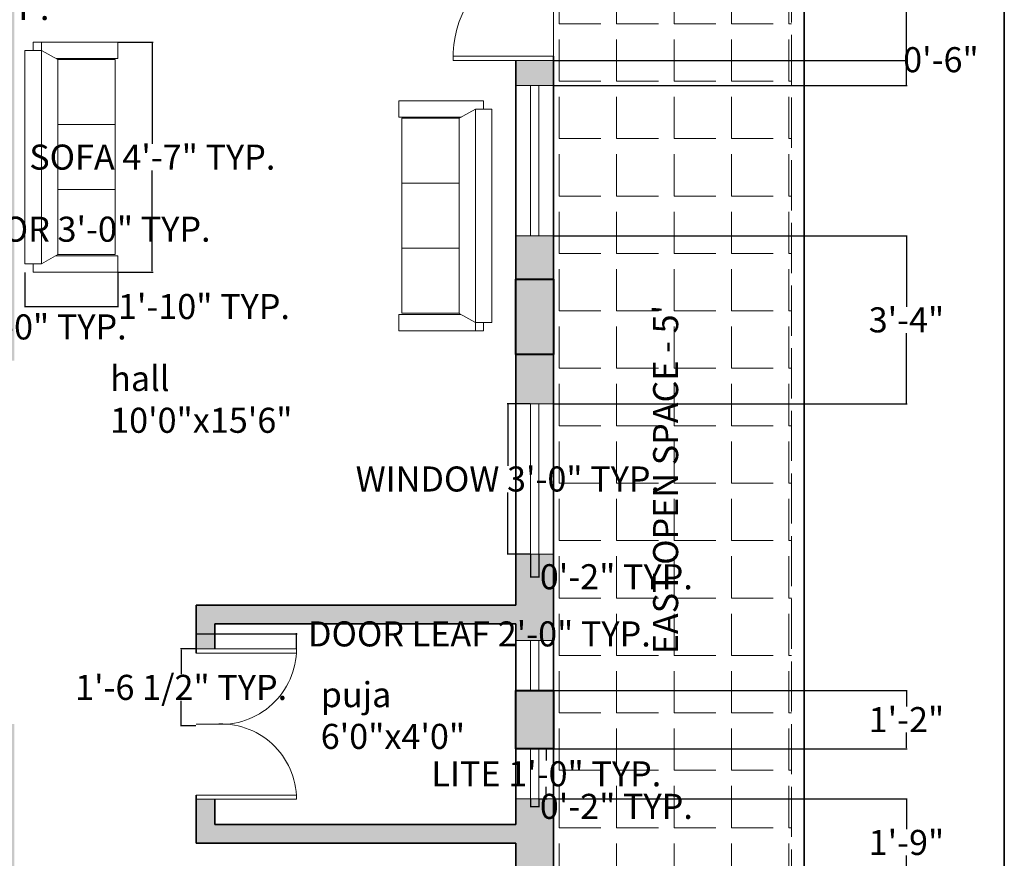
# Model space of a CAD drawing. Units: inches. Extents: x 56944 to 57417, y 173916 to 174454.
# Tile 6 of 8: x 57181 to 57417, y 174068 to 174268. Entities that reach past the tile are written whole.
import ezdxf

# ---------------------------------------------------------------- set-up
doc = ezdxf.new("R2010")
doc.units = ezdxf.units.IN
doc.header["$MEASUREMENT"] = 0
doc.linetypes.add('ACAD_ISO02W100', pattern=[15, 12, -3])
for name, color, linetype, lineweight in [('A-ANNO-DIMS', 2, 'Continuous', 18), ('A-ANNO-TEXT', 7, 'Continuous', 18), ('A-ANNO-TTLB', 7, 'Continuous', 35), ('A-AREA-IDEN', 7, 'Continuous', 20), ('A-COLS', 7, 'Continuous', 40), ('A-COLS-PATT', 250, 'Continuous', 9), ('A-DOOR', 3, 'Continuous', 20), ('A-FURN', 8, 'Continuous', 18), ('A-GLAZ', 4, 'Continuous', 18), ('A-SITE-PATT', 8, 'Continuous', 9), ('A-SITE-WALL-HIDN', 7, 'ACAD_ISO02W100', 18), ('A-WALL', 7, 'Continuous', 35), ('A-WALL-PATT', 241, 'Continuous', 9), ('C-PROP', 7, 'Continuous', 35)]:
    doc.layers.add(name, color=color, linetype=linetype, lineweight=lineweight)
doc.styles.get("Standard").update_dxf_attribs({"font": 'arial.ttf'})
doc.dimstyles.get("Standard").update_dxf_attribs({"dimtxt": 6, "dimasz": 0.18, "dimexe": 0.18, "dimexo": 0.0625, "dimgap": 0.09, "dimtad": 0, "dimtih": 1, "dimtoh": 1, "dimdec": 1, "dimzin": 0, "dimdsep": 46, "dimlunit": 3, "dimtxsty": 'Standard', "dimcen": 0.09, "dimadec": 0, "dimazin": 0, "dimtfac": 1, "dimtdec": 1, "dimtofl": 0, "dimtmove": 0, "dimatfit": 3, "dimfxl": 1, "dimtolj": 1, "dimtzin": 0, "dimarcsym": 0})

# ---------------------------------------------------------------- blocks, each defined once
blk = doc.blocks.new('SOFA-3-SEAT')
for p, q in [((1.96, 55.04), (22.23, 55.04)), ((1.96, 55.04), (1.96, 53.08)), ((3.92, 55.04), (3.92, 1.96)), ((22.23, 51.12), (22.23, 55.04)), ((0, 53.08), (0, 1.96)), ((3.92, 53.08), (0, 53.08)), ((3.92, 53.08), (7.85, 50.88)), ((7.54, 51.12), (22.23, 51.12)), ((21.57, 50.87), (7.85, 50.87)), ((21.57, 35.31), (7.85, 35.31)), ((21.57, 19.74), (7.85, 19.74)), ((7.85, 4.17), (3.92, 1.96)), ((7.28, 3.92), (22.23, 3.92)), ((22.23, 3.92), (22.23, 0)), ((3.92, 1.96), (0, 1.96)), ((1.96, 1.96), (1.96, 0)), ((1.96, 0), (22.23, 0))]:
    blk.add_line(p, q)
blk.add_lwpolyline([(7.85, 50.88), (7.85, 4.17), (21.57, 4.17), (21.57, 50.87)])
blk = doc.blocks.new('GLAZ-LITE-36IN')
for p, q in [((36, 2), (0, 2)), ((0, 0), (36, 0))]:
    blk.add_line(p, q)
blk = doc.blocks.new('GLAZ-LITE-12IN')
for p, q in [((0, 0), (0, 12)), ((2, 12), (2, 0))]:
    blk.add_line(p, q)
blk = doc.blocks.new('DOOR-PAIRED-LEAF-24IN')
for p, q in [((0, 18.06), (24, 18.06)), ((0, 18.06), (0, 17.06)), ((24, 17.06), (0, 17.06))]:
    blk.add_line(p, q)
blk.add_arc((5.94, 18.06), 18.06, 265.4188, 0)
blk = doc.blocks.new('*D14')
at = {"layer": 'A-ANNO-DIMS', "color": 0, "lineweight": -2, "transparency": 16777216}
for p, q in [((57303.07, 174176.51), (57297.55, 174176.51)), ((57297.73, 174176.33), (57297.73, 174161.7)), ((57297.73, 174140.69), (57297.73, 174155.31)), ((57303.07, 174140.51), (57297.55, 174140.51))]:
    blk.add_line(p, q, dxfattribs=at)
at = {"layer": 'A-ANNO-DIMS', "color": 0, "transparency": 16777216}
for points in [[(57297.7, 174176.33), (57297.76, 174176.33), (57297.73, 174176.51)], [(57297.7, 174140.69), (57297.76, 174140.69), (57297.73, 174140.51)]]:
    blk.add_solid(points, dxfattribs=at)
at = {"layer": 'Defpoints', "color": 0, "transparency": 16777216}
for p in [(57303.13, 174176.51), (57297.73, 174140.51), (57303.13, 174140.51)]:
    blk.add_point(p, dxfattribs=at)
at = {"layer": 'A-ANNO-DIMS', "color": 0, "transparency": 16777216, "insert": (57297.73, 174158.51), "char_height": 6, "attachment_point": 5}
blk.add_mtext('\\A1;WINDOW 3\'-0" TYP.', dxfattribs=at)
blk = doc.blocks.new('*D15')
at = {"layer": 'A-ANNO-DIMS', "color": 0, "lineweight": -2, "transparency": 16777216}
for p, q in [((57303.13, 174140.44), (57303.13, 174134.93)), ((57305.13, 174140.44), (57305.13, 174134.93)), ((57303.31, 174135.11), (57304.95, 174135.11)), ((57305.13, 174135.11), (57305.31, 174135.11))]:
    blk.add_line(p, q, dxfattribs=at)
at = {"layer": 'A-ANNO-DIMS', "color": 0, "transparency": 16777216}
for points in [[(57303.31, 174135.14), (57303.31, 174135.08), (57303.13, 174135.11)], [(57304.95, 174135.14), (57304.95, 174135.08), (57305.13, 174135.11)]]:
    blk.add_solid(points, dxfattribs=at)
at = {"layer": 'Defpoints', "color": 0, "transparency": 16777216}
for p in [(57303.13, 174140.51), (57305.13, 174140.51), (57305.13, 174135.11)]:
    blk.add_point(p, dxfattribs=at)
at = {"layer": 'A-ANNO-DIMS', "color": 0, "transparency": 16777216, "insert": (57323.69, 174135.11), "char_height": 6, "attachment_point": 5}
blk.add_mtext('\\A1;0\'-2" TYP.', dxfattribs=at)
blk = doc.blocks.new('*D16')
at = {"layer": 'A-ANNO-DIMS', "color": 0, "lineweight": -2, "transparency": 16777216}
for p, q in [((57135.34, 174305.75), (57145.76, 174305.75)), ((57145.58, 174305.57), (57145.58, 174274.59)), ((57145.58, 174237.22), (57145.58, 174268.2)), ((57135.34, 174237.04), (57145.76, 174237.04))]:
    blk.add_line(p, q, dxfattribs=at)
at = {"layer": 'A-ANNO-DIMS', "color": 0, "transparency": 16777216}
for points in [[(57145.55, 174305.57), (57145.61, 174305.57), (57145.58, 174305.75)], [(57145.55, 174237.22), (57145.61, 174237.22), (57145.58, 174237.04)]]:
    blk.add_solid(points, dxfattribs=at)
at = {"layer": 'Defpoints', "color": 0, "transparency": 16777216}
for p in [(57135.28, 174305.75), (57145.58, 174305.75), (57135.28, 174237.04)]:
    blk.add_point(p, dxfattribs=at)
at = {"layer": 'A-ANNO-DIMS', "color": 0, "transparency": 16777216, "insert": (57145.58, 174271.39), "char_height": 6, "attachment_point": 5}
blk.add_mtext('\\A1;BED SET 5\'-8 1/2" TYP.', dxfattribs=at)
blk = doc.blocks.new('*D18')
at = {"layer": 'A-ANNO-DIMS', "color": 0, "lineweight": -2, "transparency": 16777216}
for p, q in [((57204.45, 174263.1), (57212.82, 174263.1)), ((57212.64, 174262.92), (57212.64, 174238.77)), ((57212.64, 174208.24), (57212.64, 174232.38)), ((57204.45, 174208.06), (57212.82, 174208.06))]:
    blk.add_line(p, q, dxfattribs=at)
at = {"layer": 'A-ANNO-DIMS', "color": 0, "transparency": 16777216}
for points in [[(57212.61, 174262.92), (57212.67, 174262.92), (57212.64, 174263.1)], [(57212.61, 174208.24), (57212.67, 174208.24), (57212.64, 174208.06)]]:
    blk.add_solid(points, dxfattribs=at)
at = {"layer": 'Defpoints', "color": 0, "transparency": 16777216}
for p in [(57204.39, 174263.1), (57212.64, 174263.1), (57204.39, 174208.06)]:
    blk.add_point(p, dxfattribs=at)
at = {"layer": 'A-ANNO-DIMS', "color": 0, "transparency": 16777216, "insert": (57212.64, 174235.58), "char_height": 6, "attachment_point": 5}
blk.add_mtext('\\A1;SOFA 4\'-7" TYP.', dxfattribs=at)
blk = doc.blocks.new('*D19')
at = {"layer": 'A-ANNO-DIMS', "color": 0, "lineweight": -2, "transparency": 16777216}
for p, q in [((57182.16, 174207.99), (57182.16, 174199.62)), ((57204.39, 174207.99), (57204.39, 174199.62)), ((57182.34, 174199.8), (57204.21, 174199.8)), ((57204.39, 174199.8), (57204.57, 174199.8))]:
    blk.add_line(p, q, dxfattribs=at)
at = {"layer": 'A-ANNO-DIMS', "color": 0, "transparency": 16777216}
for points in [[(57182.34, 174199.83), (57182.34, 174199.77), (57182.16, 174199.8)], [(57204.21, 174199.83), (57204.21, 174199.77), (57204.39, 174199.8)]]:
    blk.add_solid(points, dxfattribs=at)
at = {"layer": 'Defpoints', "color": 0, "transparency": 16777216}
for p in [(57182.16, 174208.06), (57204.39, 174208.06), (57204.39, 174199.8)]:
    blk.add_point(p, dxfattribs=at)
at = {"layer": 'A-ANNO-DIMS', "color": 0, "transparency": 16777216, "insert": (57224.99, 174199.8), "char_height": 6, "attachment_point": 5}
blk.add_mtext('\\A1;1\'-10" TYP.', dxfattribs=at)
blk = doc.blocks.new('*D22')
at = {"layer": 'A-ANNO-DIMS', "color": 0, "lineweight": -2, "transparency": 16777216}
for p, q in [((57169.7, 174236.32), (57175.21, 174236.32)), ((57175.03, 174236.14), (57175.03, 174221.52)), ((57175.03, 174200.5), (57175.03, 174215.13)), ((57169.7, 174200.32), (57175.21, 174200.32))]:
    blk.add_line(p, q, dxfattribs=at)
at = {"layer": 'A-ANNO-DIMS', "color": 0, "transparency": 16777216}
for points in [[(57175, 174236.14), (57175.06, 174236.14), (57175.03, 174236.32)], [(57175, 174200.5), (57175.06, 174200.5), (57175.03, 174200.32)]]:
    blk.add_solid(points, dxfattribs=at)
at = {"layer": 'Defpoints', "color": 0, "transparency": 16777216}
for p in [(57169.63, 174236.32), (57175.03, 174236.32), (57169.63, 174200.32)]:
    blk.add_point(p, dxfattribs=at)
at = {"layer": 'A-ANNO-DIMS', "color": 0, "transparency": 16777216, "insert": (57175.03, 174218.32), "char_height": 6, "attachment_point": 5}
blk.add_mtext('\\A1;BEDROOM DOOR 3\'-0" TYP.', dxfattribs=at)
blk = doc.blocks.new('*D23')
at = {"layer": 'A-ANNO-DIMS', "color": 0, "lineweight": -2, "transparency": 16777216}
for p, q in [((57133.63, 174200.26), (57133.63, 174194.74)), ((57169.63, 174200.26), (57169.63, 174194.74)), ((57133.81, 174194.92), (57169.45, 174194.92)), ((57169.63, 174194.92), (57169.81, 174194.92))]:
    blk.add_line(p, q, dxfattribs=at)
at = {"layer": 'A-ANNO-DIMS', "color": 0, "transparency": 16777216}
for points in [[(57133.81, 174194.95), (57133.81, 174194.89), (57133.63, 174194.92)], [(57169.45, 174194.95), (57169.45, 174194.89), (57169.63, 174194.92)]]:
    blk.add_solid(points, dxfattribs=at)
at = {"layer": 'Defpoints', "color": 0, "transparency": 16777216}
for p in [(57133.63, 174200.32), (57169.63, 174200.32), (57169.63, 174194.92)]:
    blk.add_point(p, dxfattribs=at)
at = {"layer": 'A-ANNO-DIMS', "color": 0, "transparency": 16777216, "insert": (57188.19, 174194.92), "char_height": 6, "attachment_point": 5}
blk.add_mtext('\\A1;3\'-0" TYP.', dxfattribs=at)
blk = doc.blocks.new('*D28')
at = {"layer": 'A-ANNO-DIMS', "color": 0, "lineweight": -2, "transparency": 16777216}
for p, q in [((57305.2, 174093.93), (57307.11, 174093.93)), ((57306.93, 174093.75), (57306.93, 174091.08)), ((57306.93, 174082.11), (57306.93, 174084.78)), ((57305.2, 174081.93), (57307.11, 174081.93))]:
    blk.add_line(p, q, dxfattribs=at)
at = {"layer": 'A-ANNO-DIMS', "color": 0, "transparency": 16777216}
for points in [[(57306.9, 174093.75), (57306.96, 174093.75), (57306.93, 174093.93)], [(57306.9, 174082.11), (57306.96, 174082.11), (57306.93, 174081.93)]]:
    blk.add_solid(points, dxfattribs=at)
at = {"layer": 'Defpoints', "color": 0, "transparency": 16777216}
for p in [(57305.13, 174093.93), (57306.93, 174093.93), (57305.13, 174081.93)]:
    blk.add_point(p, dxfattribs=at)
at = {"layer": 'A-ANNO-DIMS', "color": 0, "transparency": 16777216, "insert": (57306.93, 174087.93), "char_height": 6, "attachment_point": 5}
blk.add_mtext('\\A1;LITE 1\'-0" TYP.', dxfattribs=at)
blk = doc.blocks.new('*D29')
at = {"layer": 'A-ANNO-DIMS', "color": 0, "lineweight": -2, "transparency": 16777216}
for p, q in [((57303.13, 174081.87), (57303.13, 174079.95)), ((57303.31, 174080.13), (57304.95, 174080.13)), ((57305.13, 174081.87), (57305.13, 174079.95)), ((57305.13, 174080.13), (57305.31, 174080.13))]:
    blk.add_line(p, q, dxfattribs=at)
at = {"layer": 'A-ANNO-DIMS', "color": 0, "transparency": 16777216}
for points in [[(57303.31, 174080.16), (57303.31, 174080.1), (57303.13, 174080.13)], [(57304.95, 174080.16), (57304.95, 174080.1), (57305.13, 174080.13)]]:
    blk.add_solid(points, dxfattribs=at)
at = {"layer": 'Defpoints', "color": 0, "transparency": 16777216}
for p in [(57303.13, 174081.93), (57305.13, 174081.93), (57305.13, 174080.13)]:
    blk.add_point(p, dxfattribs=at)
at = {"layer": 'A-ANNO-DIMS', "color": 0, "transparency": 16777216, "insert": (57323.69, 174080.13), "char_height": 6, "attachment_point": 5}
blk.add_mtext('\\A1;0\'-2" TYP.', dxfattribs=at)
blk = doc.blocks.new('*D30')
at = {"layer": 'A-ANNO-DIMS', "color": 0, "lineweight": -2, "transparency": 16777216}
for p, q in [((57223.13, 174117.89), (57223.13, 174121.6)), ((57223.31, 174121.42), (57246.95, 174121.42)), ((57247.13, 174117.89), (57247.13, 174121.6)), ((57247.13, 174121.42), (57247.31, 174121.42))]:
    blk.add_line(p, q, dxfattribs=at)
at = {"layer": 'A-ANNO-DIMS', "color": 0, "transparency": 16777216}
for points in [[(57223.31, 174121.45), (57223.31, 174121.39), (57223.13, 174121.42)], [(57246.95, 174121.45), (57246.95, 174121.39), (57247.13, 174121.42)]]:
    blk.add_solid(points, dxfattribs=at)
at = {"layer": 'Defpoints', "color": 0, "transparency": 16777216}
for p in [(57247.13, 174121.42), (57223.13, 174117.82), (57247.13, 174117.82)]:
    blk.add_point(p, dxfattribs=at)
at = {"layer": 'A-ANNO-DIMS', "color": 0, "transparency": 16777216, "insert": (57290.92, 174121.42), "char_height": 6, "attachment_point": 5}
blk.add_mtext('\\A1;DOOR LEAF 2\'-0" TYP.', dxfattribs=at)
blk = doc.blocks.new('*D31')
at = {"layer": 'A-ANNO-DIMS', "color": 0, "lineweight": -2, "transparency": 16777216}
for p, q in [((57223.07, 174117.82), (57219.35, 174117.82)), ((57219.53, 174117.64), (57219.53, 174111.81)), ((57219.53, 174099.6), (57219.53, 174105.43)), ((57223.07, 174099.42), (57219.35, 174099.42))]:
    blk.add_line(p, q, dxfattribs=at)
at = {"layer": 'A-ANNO-DIMS', "color": 0, "transparency": 16777216}
for points in [[(57219.5, 174117.64), (57219.56, 174117.64), (57219.53, 174117.82)], [(57219.5, 174099.6), (57219.56, 174099.6), (57219.53, 174099.42)]]:
    blk.add_solid(points, dxfattribs=at)
at = {"layer": 'Defpoints', "color": 0, "transparency": 16777216}
for p in [(57219.53, 174117.82), (57223.13, 174117.82), (57223.13, 174099.42)]:
    blk.add_point(p, dxfattribs=at)
at = {"layer": 'A-ANNO-DIMS', "color": 0, "transparency": 16777216, "insert": (57219.53, 174108.62), "char_height": 6, "attachment_point": 5}
blk.add_mtext('\\A1;1\'-6 1/2" TYP.', dxfattribs=at)
blk = doc.blocks.new('*D45')
at = {"layer": 'A-ANNO-DIMS', "color": 0, "lineweight": -2, "transparency": 16777216}
for p, q in [((57308.7, 174306.82), (57393.31, 174306.82)), ((57393.13, 174306.64), (57393.13, 174285.93)), ((57393.13, 174258.9), (57393.13, 174279.62)), ((57308.7, 174258.72), (57393.31, 174258.72))]:
    blk.add_line(p, q, dxfattribs=at)
at = {"layer": 'A-ANNO-DIMS', "color": 0, "transparency": 16777216}
for points in [[(57393.1, 174306.64), (57393.16, 174306.64), (57393.13, 174306.82)], [(57393.1, 174258.9), (57393.16, 174258.9), (57393.13, 174258.72)]]:
    blk.add_solid(points, dxfattribs=at)
at = {"layer": 'Defpoints', "color": 0, "transparency": 16777216}
for p in [(57308.63, 174306.82), (57393.13, 174306.82), (57308.63, 174258.72)]:
    blk.add_point(p, dxfattribs=at)
at = {"layer": 'A-ANNO-DIMS', "color": 0, "transparency": 16777216, "insert": (57393.13, 174282.77), "char_height": 6, "attachment_point": 5}
blk.add_mtext('\\A1;4\'-0"', dxfattribs=at)
blk = doc.blocks.new('*D50')
at = {"layer": 'A-ANNO-DIMS', "color": 0, "lineweight": -2, "transparency": 16777216}
for p, q in [((57308.7, 174081.93), (57393.31, 174081.93)), ((57393.13, 174081.75), (57393.13, 174074.65)), ((57393.13, 174061.23), (57393.13, 174068.34)), ((57308.7, 174061.05), (57393.31, 174061.05))]:
    blk.add_line(p, q, dxfattribs=at)
at = {"layer": 'A-ANNO-DIMS', "color": 0, "transparency": 16777216}
for points in [[(57393.1, 174081.75), (57393.16, 174081.75), (57393.13, 174081.93)], [(57393.1, 174061.23), (57393.16, 174061.23), (57393.13, 174061.05)]]:
    blk.add_solid(points, dxfattribs=at)
at = {"layer": 'Defpoints', "color": 0, "transparency": 16777216}
for p in [(57308.63, 174081.93), (57393.13, 174081.93), (57308.63, 174061.05)]:
    blk.add_point(p, dxfattribs=at)
at = {"layer": 'A-ANNO-DIMS', "color": 0, "transparency": 16777216, "insert": (57393.13, 174071.49), "char_height": 6, "attachment_point": 5}
blk.add_mtext('\\A1;1\'-9"', dxfattribs=at)
blk = doc.blocks.new('*D51')
at = {"layer": 'A-ANNO-DIMS', "color": 0, "lineweight": -2, "transparency": 16777216}
for p, q in [((57308.7, 174107.87), (57393.31, 174107.87)), ((57393.13, 174107.69), (57393.13, 174104)), ((57393.13, 174094.11), (57393.13, 174097.8)), ((57308.7, 174093.93), (57393.31, 174093.93))]:
    blk.add_line(p, q, dxfattribs=at)
at = {"layer": 'A-ANNO-DIMS', "color": 0, "transparency": 16777216}
for points in [[(57393.1, 174107.69), (57393.16, 174107.69), (57393.13, 174107.87)], [(57393.1, 174094.11), (57393.16, 174094.11), (57393.13, 174093.93)]]:
    blk.add_solid(points, dxfattribs=at)
at = {"layer": 'Defpoints', "color": 0, "transparency": 16777216}
for p in [(57308.63, 174107.87), (57393.13, 174107.87), (57308.63, 174093.93)]:
    blk.add_point(p, dxfattribs=at)
at = {"layer": 'A-ANNO-DIMS', "color": 0, "transparency": 16777216, "insert": (57393.13, 174100.9), "char_height": 6, "attachment_point": 5}
blk.add_mtext('\\A1;1\'-2"', dxfattribs=at)
blk = doc.blocks.new('*D52')
at = {"layer": 'A-ANNO-DIMS', "color": 0, "lineweight": -2, "transparency": 16777216}
for p, q in [((57308.7, 174258.72), (57393.31, 174258.72)), ((57393.13, 174258.72), (57393.13, 174258.9)), ((57393.13, 174258.9), (57393.31, 174258.9)), ((57393.13, 174252.9), (57393.13, 174258.54)), ((57308.7, 174252.72), (57393.31, 174252.72))]:
    blk.add_line(p, q, dxfattribs=at)
at = {"layer": 'A-ANNO-DIMS', "color": 0, "transparency": 16777216}
for points in [[(57393.1, 174258.54), (57393.16, 174258.54), (57393.13, 174258.72)], [(57393.1, 174252.9), (57393.16, 174252.9), (57393.13, 174252.72)]]:
    blk.add_solid(points, dxfattribs=at)
at = {"layer": 'Defpoints', "color": 0, "transparency": 16777216}
for p in [(57308.63, 174258.72), (57393.13, 174258.72), (57308.63, 174252.72)]:
    blk.add_point(p, dxfattribs=at)
at = {"layer": 'A-ANNO-DIMS', "color": 0, "transparency": 16777216, "insert": (57401.38, 174258.9), "char_height": 6, "attachment_point": 5}
blk.add_mtext('\\A1;0\'-6"', dxfattribs=at)
blk = doc.blocks.new('*D53')
at = {"layer": 'A-ANNO-DIMS', "color": 0, "lineweight": -2, "transparency": 16777216}
for p, q in [((57308.7, 174216.72), (57393.31, 174216.72)), ((57393.13, 174216.54), (57393.13, 174199.77)), ((57393.13, 174176.69), (57393.13, 174193.46)), ((57308.7, 174176.51), (57393.31, 174176.51))]:
    blk.add_line(p, q, dxfattribs=at)
at = {"layer": 'A-ANNO-DIMS', "color": 0, "transparency": 16777216}
for points in [[(57393.1, 174216.54), (57393.16, 174216.54), (57393.13, 174216.72)], [(57393.1, 174176.69), (57393.16, 174176.69), (57393.13, 174176.51)]]:
    blk.add_solid(points, dxfattribs=at)
at = {"layer": 'Defpoints', "color": 0, "transparency": 16777216}
for p in [(57308.63, 174216.72), (57393.13, 174216.72), (57308.63, 174176.51)]:
    blk.add_point(p, dxfattribs=at)
at = {"layer": 'A-ANNO-DIMS', "color": 0, "transparency": 16777216, "insert": (57393.13, 174196.61), "char_height": 6, "attachment_point": 5}
blk.add_mtext('\\A1;3\'-4"', dxfattribs=at)

msp = doc.modelspace()

# ---------------------------------------------------------------- hatches: boundary and pattern name
at = {"layer": 'A-COLS-PATT'}
h = msp.add_hatch(color=256, dxfattribs=at)
h.dxf.hatch_style = 1
h.paths.add_polyline_path([(57052.13, 174321.82), (57034.13, 174321.82), (57034.13, 174312.82), (57052.13, 174312.82)])
h.paths.add_polyline_path([(57186.38, 174321.82), (57168.38, 174321.82), (57168.38, 174312.82), (57175.13, 174312.82), (57186.38, 174312.82)])
h.paths.add_polyline_path([(57308.63, 174321.82), (57290.63, 174321.82), (57290.63, 174312.82), (57308.63, 174312.82)])
h.paths.add_polyline_path([(57179.63, 174204.82), (57170.63, 174204.82), (57170.63, 174186.82), (57179.63, 174186.82)])
h.paths.add_polyline_path([(57043.13, 174204.82), (57034.13, 174204.82), (57034.13, 174186.82), (57043.13, 174186.82)])
h.paths.add_polyline_path([(57308.63, 174206.32), (57299.63, 174206.32), (57299.63, 174188.32), (57308.63, 174188.32)])
h.paths.add_polyline_path([(57308.63, 174107.87), (57299.63, 174107.87), (57299.63, 174093.93), (57308.63, 174093.93)])
h.paths.add_polyline_path([(57308.63, 173978.32), (57299.63, 173978.32), (57299.63, 173960.32), (57308.63, 173960.32)])
h.paths.add_polyline_path([(57179.63, 173969.32), (57161.63, 173969.32), (57161.63, 173960.32), (57179.63, 173960.32)])
h.paths.add_polyline_path([(57043.13, 173978.32), (57034.13, 173978.32), (57034.13, 173960.32), (57043.13, 173960.32)])
h.paths.add_polyline_path([(57043.13, 174099.82), (57034.13, 174099.82), (57034.13, 174081.82), (57043.13, 174081.82)])
h.paths.add_polyline_path([(57179.63, 174099.82), (57170.63, 174099.82), (57170.63, 174081.82), (57179.63, 174081.82)])
at = {"layer": 'A-SITE-PATT'}
h = msp.add_hatch(dxfattribs=at)
h.set_pattern_fill('ANGLE', color=256, scale=50)
h.set_pattern_definition([(0, (0, 0), (0, 13.75), [10, -3.75]), (90, (0, 0), (-13.75, 8e-16), [10, -3.75])])
h.paths.add_polyline_path([(57365.63, 174396.82), (57200.13, 174396.82), (57200.13, 174379.18), (57215.46, 174379.18, -1.049383), (57218.84, 174379.34, -0.952941), (57215.46, 174379.18), (57200.13, 174379.18), (57200.13, 174360.82), (57140.13, 174360.82), (57140.13, 174321.82), (57149.42, 174321.82), (57243.2, 174321.82), (57282.32, 174321.82), (57283.32, 174321.82), (57308.63, 174321.82), (57308.63, 174305.82), (57308.63, 174259.72), (57308.63, 174258.72), (57308.63, 174252.72), (57308.63, 174216.72), (57308.63, 174099.82), (57308.63, 174093.93), (57308.63, 174081.93), (57308.63, 173969.32), (57365.63, 173969.32)])
h.paths.add_polyline_path([(57341.88, 174114.38), (57341.88, 174209.81), (57329.51, 174209.81), (57329.51, 174114.38)], flags=24)
h.paths.add_polyline_path([(57215.63, 174350.61), (57326.6, 174350.61), (57326.6, 174362.97), (57215.63, 174362.97)], flags=24)
at = {"layer": 'A-WALL-PATT'}
h = msp.add_hatch(color=256, dxfattribs=at)
h.dxf.hatch_style = 1
h.paths.add_polyline_path([(57089.42, 174321.82), (57052.13, 174321.82), (57052.13, 174312.82), (57089.42, 174312.82)])
h.paths.add_polyline_path([(57168.38, 174321.82), (57149.42, 174321.82), (57149.42, 174312.82), (57168.38, 174312.82)])
h.paths.add_polyline_path([(57199.66, 174321.82), (57186.38, 174321.82), (57186.38, 174312.82), (57199.66, 174312.82)])
h.paths.add_polyline_path([(57179.63, 174312.82), (57177.38, 174312.82), (57175.13, 174312.82), (57175.13, 174204.82), (57179.63, 174204.82)])
h.paths.add_polyline_path([(57043.13, 174312.82), (57034.13, 174312.82), (57034.13, 174204.82), (57043.13, 174204.82)])
h.paths.add_polyline_path([(57043.13, 174147.82), (57121.13, 174147.82), (57121.13, 174099.82), (57115.13, 174099.82), (57115.13, 174095.32), (57121.13, 174095.32), (57133.63, 174095.32), (57133.63, 174099.82), (57125.63, 174099.82), (57125.63, 174200.32), (57133.63, 174200.32), (57133.63, 174204.82), (57115.13, 174204.82), (57115.13, 174200.32), (57121.13, 174200.32), (57121.13, 174152.32), (57043.13, 174152.32), (57043.13, 174162.82), (57034.13, 174162.82), (57034.13, 174131.11), (57043.13, 174131.11)])
h.paths.add_polyline_path([(57043.13, 174081.82), (57034.13, 174081.82), (57034.13, 173978.32), (57043.13, 173978.32)])
h.paths.add_polyline_path([(57093.93, 173969.32), (57043.13, 173969.32), (57043.13, 173960.32), (57093.93, 173960.32)])
h.paths.add_polyline_path([(57161.63, 173969.32), (57153.93, 173969.32), (57153.93, 173960.32), (57161.63, 173960.32)])
h.paths.add_polyline_path([(57179.63, 174081.82), (57175.13, 174081.82), (57175.13, 173969.32), (57179.63, 173969.32)])
h.paths.add_polyline_path([(57299.63, 173969.32), (57179.63, 173969.32), (57179.63, 173960.32), (57299.63, 173960.32)])
h.paths.add_polyline_path([(57308.63, 174025.05), (57299.63, 174025.05), (57299.63, 173978.32), (57308.63, 173978.32)])
h.paths.add_polyline_path([(57308.63, 174081.93), (57299.63, 174081.93), (57299.63, 174075.82), (57227.63, 174075.82), (57227.63, 174081.82), (57223.13, 174081.82), (57223.13, 174075.82), (57223.13, 174071.32), (57299.63, 174071.32), (57299.63, 174061.05), (57308.63, 174061.05)])
h.paths.add_polyline_path([(57308.63, 174140.51), (57299.63, 174140.51), (57299.63, 174128.32), (57223.13, 174128.32), (57223.13, 174117.82), (57227.63, 174117.82), (57227.63, 174123.82), (57299.63, 174123.82), (57299.63, 174119.87), (57308.63, 174119.87)])
h.paths.add_polyline_path([(57308.63, 174216.72), (57299.63, 174216.72), (57299.63, 174206.32), (57308.63, 174206.32)])
h.paths.add_polyline_path([(57308.63, 174188.32), (57299.63, 174188.32), (57299.63, 174176.51), (57308.63, 174176.51)])
h.paths.add_polyline_path([(57308.63, 174258.72), (57299.63, 174258.72), (57299.63, 174252.72), (57308.63, 174252.72)])
h.paths.add_polyline_path([(57308.63, 174312.82), (57299.63, 174312.82), (57299.63, 174306.82), (57308.63, 174306.82)])
h.paths.add_polyline_path([(57290.63, 174321.82), (57283.32, 174321.82), (57283.32, 174312.82), (57290.63, 174312.82)])
h.paths.add_polyline_path([(57242.2, 174321.82), (57235.66, 174321.82), (57235.66, 174312.82), (57242.2, 174312.82)])
h.paths.add_polyline_path([(57083.13, 174204.82), (57043.13, 174204.82), (57043.13, 174200.32), (57083.13, 174200.32)], flags=17)
h.paths.add_polyline_path([(57083.13, 174099.82), (57043.13, 174099.82), (57043.13, 174095.32), (57083.13, 174095.32)], flags=0)

# ---------------------------------------------------------------- linework, layer by layer
at = {"layer": 'A-ANNO-TTLB'}
msp.add_lwpolyline([(56943.57, 174453.61), (57416.55, 174453.61), (57416.55, 173915.6), (56943.57, 173915.6)], close=True, dxfattribs=at)
at = {"layer": 'A-COLS'}
for p, q in [((57299.63, 174206.32), (57308.63, 174206.32)), ((57299.63, 174188.32), (57299.63, 174206.32)), ((57308.63, 174206.32), (57308.63, 174188.32)), ((57308.63, 174188.32), (57299.63, 174188.32)), ((57299.63, 174107.87), (57308.63, 174107.87)), ((57299.63, 174093.93), (57299.63, 174107.87)), ((57308.63, 174107.87), (57308.63, 174093.93)), ((57308.63, 174093.93), (57299.63, 174093.93)), ((57299.63, 174093.93), (57299.63, 174093.93))]:
    msp.add_line(p, q, dxfattribs=at)
at = {"layer": 'A-DOOR'}
for p, q in [((57308.63, 174305.82), (57308.63, 174259.72)), ((57284.63, 174259.72), (57308.63, 174259.72)), ((57308.63, 174258.72), (57308.63, 174259.72)), ((57308.63, 174258.72), (57284.63, 174258.72)), ((57284.63, 174258.72), (57308.63, 174258.72)), ((57247.13, 174117.82), (57223.13, 174117.82)), ((57223.13, 174116.82), (57223.13, 174117.82)), ((57223.13, 174099.82), (57227.63, 174099.82)), ((57247.13, 174081.82), (57223.13, 174081.82))]:
    msp.add_line(p, q, dxfattribs=at)
msp.add_arc((57310.15, 174259.51), 25.53, 114.3285, 181.7674, dxfattribs=at)
at = {"layer": 'A-GLAZ'}
for p, q in [((57308.63, 174252.72), (57299.63, 174252.72)), ((57299.63, 174252.72), (57299.63, 174216.72)), ((57308.63, 174216.72), (57308.63, 174252.72)), ((57299.63, 174216.72), (57308.63, 174216.72)), ((57299.63, 174140.51), (57299.63, 174176.51)), ((57299.63, 174176.51), (57308.63, 174176.51)), ((57308.63, 174176.51), (57308.63, 174140.51)), ((57308.63, 174140.51), (57299.63, 174140.51)), ((57299.63, 174107.87), (57299.63, 174119.87)), ((57299.63, 174119.87), (57308.63, 174119.87)), ((57308.63, 174119.87), (57308.63, 174107.87)), ((57308.63, 174107.87), (57299.63, 174107.87)), ((57299.63, 174093.93), (57308.63, 174093.93)), ((57299.63, 174081.93), (57299.63, 174093.93)), ((57308.63, 174093.93), (57308.63, 174081.93)), ((57308.63, 174081.93), (57299.63, 174081.93))]:
    msp.add_line(p, q, dxfattribs=at)
at = {"layer": 'A-SITE-WALL-HIDN'}
msp.add_line((57365.63, 174399.82), (57365.63, 173969.32), dxfattribs=at)
at = {"layer": 'A-WALL'}
for p, q in [((57308.63, 174259.72), (57308.63, 174099.82)), ((57299.63, 174258.72), (57299.63, 174128.32)), ((57308.63, 174252.72), (57308.63, 174258.72)), ((57223.13, 174128.32), (57223.13, 174116.82)), ((57223.13, 174128.32), (57299.63, 174128.32)), ((57223.13, 174123.82), (57223.13, 174117.82)), ((57227.63, 174123.82), (57227.63, 174117.82)), ((57227.63, 174123.82), (57299.63, 174123.82)), ((57299.63, 174123.82), (57299.63, 174099.82)), ((57299.63, 174099.82), (57299.63, 174075.82)), ((57308.63, 174099.82), (57308.63, 173960.32)), ((57223.13, 174082.82), (57223.13, 174071.32)), ((57223.13, 174075.82), (57223.13, 174081.82)), ((57227.63, 174081.82), (57227.63, 174075.82)), ((57227.63, 174075.82), (57299.63, 174075.82)), ((57223.13, 174071.32), (57299.63, 174071.32)), ((57299.63, 174071.32), (57299.63, 173960.32))]:
    msp.add_line(p, q, dxfattribs=at)
at = {"layer": 'C-PROP'}
msp.add_line((57368.63, 174399.82), (57368.63, 173960.32), dxfattribs=at)

# ---------------------------------------------------------------- block references
at = {"layer": 'A-DOOR'}
msp.add_blockref('DOOR-PAIRED-LEAF-24IN', (57223.13, 174099.77), dxfattribs=at)
at = {"layer": 'A-DOOR', "extrusion": (0, 0, -1), "zscale": -1, "rotation": 180}
msp.add_blockref('DOOR-PAIRED-LEAF-24IN', (-57223.13, 174099.88), dxfattribs=at)
at = {"layer": 'A-FURN'}
msp.add_blockref('SOFA-3-SEAT', (57182.16, 174208.06), dxfattribs=at)
at = {"layer": 'A-FURN', "rotation": 180}
msp.add_blockref('SOFA-3-SEAT', (57293.9, 174249.05), dxfattribs=at)
at = {"layer": 'A-GLAZ'}
for p, rotation in [((57303.13, 174252.72), 270.0000000000436), ((57303.13, 174176.51), 270.0000000000256)]:
    msp.add_blockref('GLAZ-LITE-36IN', p, dxfattribs=dict(at, rotation=rotation))
for p in [(57303.13, 174107.87), (57303.13, 174081.93)]:
    msp.add_blockref('GLAZ-LITE-12IN', p, dxfattribs=at)

# ---------------------------------------------------------------- texts
at = {"layer": 'A-ANNO-TEXT', "insert": (57332.49, 174116.55), "char_height": 6, "attachment_point": 1, "rotation": 90}
msp.add_mtext_dynamic_manual_height_columns("EAST OPEN SPACE - 5'", width=219.5086, gutter_width=1, heights=[0], dxfattribs=at)
at = {"layer": 'A-AREA-IDEN', "char_height": 6, "attachment_point": 1}
for s, width, insert in [('hall\\P10\'0"x15\'6"', 66.1923, (57202.54, 174185.57)), ('puja\\P6\'0"x4\'0"', 40.7375, (57252.94, 174109.88))]:
    msp.add_mtext_dynamic_manual_height_columns(s, width=width, gutter_width=1, heights=[0], dxfattribs=dict(at, insert=insert))

# ---------------------------------------------------------------- dimensions: what is measured, and where the dimension line sits
at = {"layer": 'A-ANNO-DIMS'}
for base, p1, p2, picture, middle in [((57393.13, 174306.82), (57308.63, 174258.72), (57308.63, 174306.82), '*D45', (57393.13, 174282.77)), ((57393.13, 174258.72), (57308.63, 174252.72), (57308.63, 174258.72), '*D52', (57401.38, 174258.9)), ((57393.13, 174216.72), (57308.63, 174176.51), (57308.63, 174216.72), '*D53', (57393.13, 174196.61)), ((57393.13, 174107.87), (57308.63, 174093.93), (57308.63, 174107.87), '*D51', (57393.13, 174100.9)), ((57393.13, 174081.93), (57308.63, 174061.05), (57308.63, 174081.93), '*D50', (57393.13, 174071.49))]:
    dim = msp.add_linear_dim(base=base, p1=p1, p2=p2, angle=90, dimstyle='Standard', override={"dimdec": 1, "dimlfac": 1, "dimrnd": 0, "dimzin": 1, "dimdsep": 46, "dimlunit": 4, "dimfrac": 2}, dxfattribs=at)
    dim.commit()
    dim.dimension.update_dxf_attribs({"geometry": picture, "text_midpoint": middle})
for base, p1, p2, angle, text, picture, middle in [((57145.58, 174305.75), (57135.28, 174237.04), (57135.28, 174305.75), 90, 'BED SET <> TYP.', '*D16', (57145.58, 174271.39)), ((57212.64, 174263.1), (57204.39, 174208.06), (57204.39, 174263.1), 90, 'SOFA <> TYP.', '*D18', (57212.64, 174235.58)), ((57175.03, 174236.32), (57169.63, 174200.32), (57169.63, 174236.32), 90, 'BEDROOM DOOR <> TYP.', '*D22', (57175.03, 174218.32)), ((57297.73, 174140.51), (57303.13, 174176.51), (57303.13, 174140.51), 270, 'WINDOW <> TYP.', '*D14', (57297.73, 174158.51)), ((57219.53, 174117.82), (57223.13, 174099.42), (57223.13, 174117.82), 90, '<> TYP.', '*D31', (57219.53, 174108.62)), ((57306.93, 174093.93), (57305.13, 174081.93), (57305.13, 174093.93), 90, 'LITE <> TYP.', '*D28', (57306.93, 174087.93))]:
    dim = msp.add_linear_dim(base=base, p1=p1, p2=p2, angle=angle, text=text, dimstyle='Standard', override={"dimdec": 1, "dimlfac": 1, "dimrnd": 0, "dimzin": 1, "dimdsep": 46, "dimlunit": 4, "dimfrac": 2}, dxfattribs=at)
    dim.commit()
    dim.dimension.update_dxf_attribs({"geometry": picture, "text_midpoint": middle})
for base, p1, p2, text, picture, middle in [((57204.39, 174199.8), (57182.16, 174208.06), (57204.39, 174208.06), '<> TYP.', '*D19', (57224.99, 174199.8)), ((57169.63, 174194.92), (57133.63, 174200.32), (57169.63, 174200.32), '<> TYP.', '*D23', (57188.19, 174194.92)), ((57305.13, 174135.11), (57303.13, 174140.51), (57305.13, 174140.51), '<> TYP.', '*D15', (57323.69, 174135.11)), ((57247.13, 174121.42), (57223.13, 174117.82), (57247.13, 174117.82), 'DOOR LEAF <> TYP.', '*D30', (57290.92, 174121.42)), ((57305.13, 174080.13), (57303.13, 174081.93), (57305.13, 174081.93), '<> TYP.', '*D29', (57323.69, 174080.13))]:
    dim = msp.add_linear_dim(base=base, p1=p1, p2=p2, text=text, dimstyle='Standard', override={"dimdec": 1, "dimlfac": 1, "dimrnd": 0, "dimzin": 1, "dimdsep": 46, "dimlunit": 4, "dimfrac": 2}, dxfattribs=at)
    dim.commit()
    dim.dimension.update_dxf_attribs({"geometry": picture, "text_midpoint": middle})

doc.saveas('drawing.dxf')
